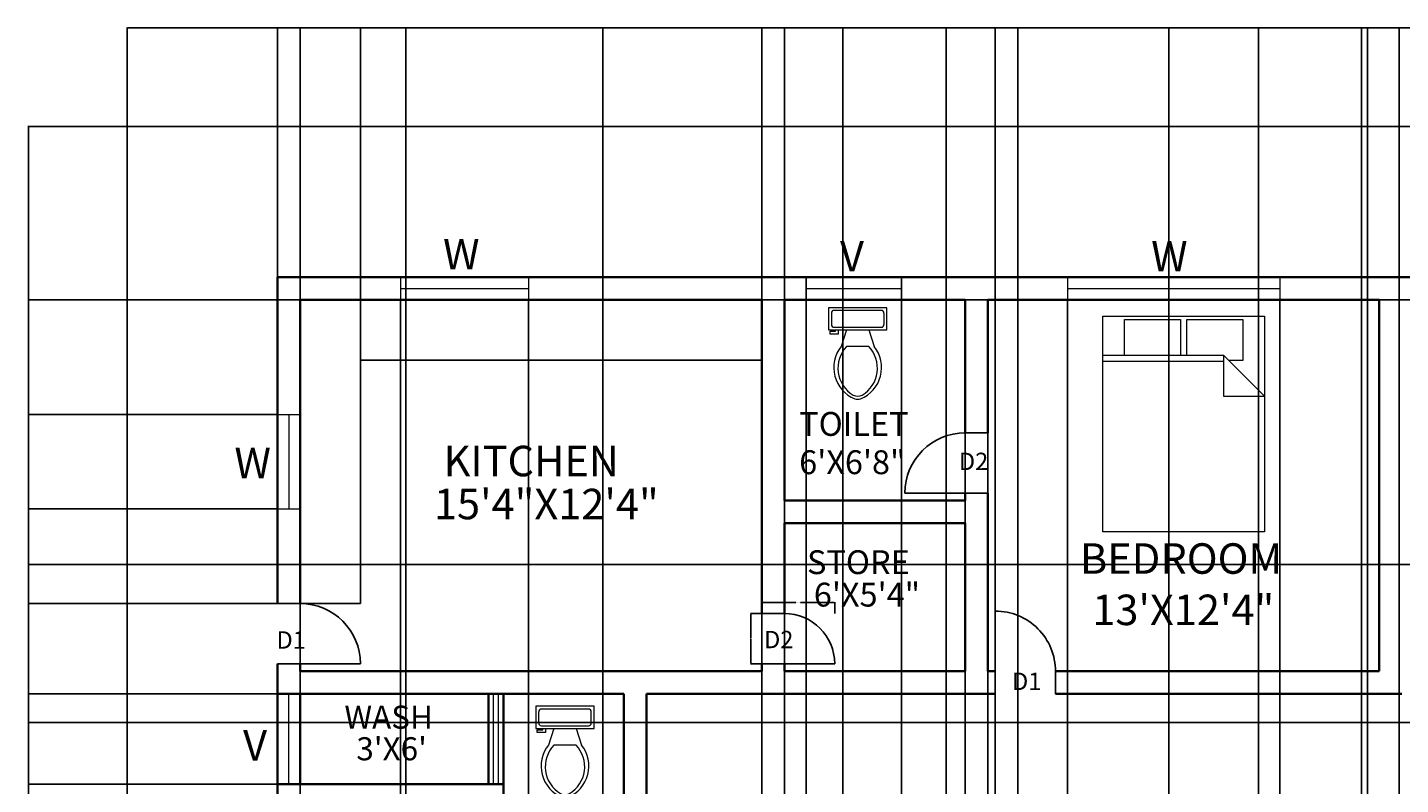
# Model space of a CAD drawing. Units: feet. Extents: x 2270 to 3094, y 1543 to 2352.
# Tile 5 of 6: x 2270 to 2817, y 2050 to 2352. Entities that reach past the tile are written whole.
import ezdxf

# ---------------------------------------------------------------- set-up
doc = ezdxf.new("R2010")
doc.units = ezdxf.units.FT
for name, color, linetype, lineweight in [('A-ANNO-DIMS', 2, 'Continuous', 18), ('A-ANNO-TEXT', 7, 'Continuous', 18), ('A-AREA-IDEN', 7, 'Continuous', 18), ('A-DOOR', 3, 'Continuous', 25), ('A-FLOR-CASE', 8, 'Continuous', 25), ('A-FLOR-FIXT', 8, 'Continuous', 18), ('A-FURN', 8, 'Continuous', 18), ('A-GLAZ', 4, 'Continuous', 18), ('A-WALL', 7, 'Continuous', 35), ('C-PROP', 8, 'Continuous', 25)]:
    doc.layers.add(name, color=color, linetype=linetype, lineweight=lineweight)
doc.styles.get("Standard").update_dxf_attribs({"font": 'arial.ttf'})
doc.dimstyles.get("Standard").update_dxf_attribs({"dimtxt": 0.18, "dimasz": 0.18, "dimexe": 0.18, "dimexo": 0.0625, "dimgap": 0.09, "dimtad": 0, "dimtih": 1, "dimtoh": 1, "dimdec": 4, "dimzin": 0, "dimdsep": 46, "dimtxsty": 'Standard', "dimcen": 0.09, "dimadec": 0, "dimazin": 0, "dimtfac": 1, "dimtdec": 4, "dimtofl": 0, "dimtmove": 0, "dimatfit": 3, "dimfxl": 1, "dimtolj": 1, "dimtzin": 0, "dimarcsym": 0})

# ---------------------------------------------------------------- blocks, each defined once
blk = doc.blocks.new('Bed - Queen')
for p, q in [((0, -80.00003), (0, 0)), ((0, 0), (59.99999, 0)), ((59.99999, 0), (59.99999, -80.00003)), ((7.99999, -1.2), (28.79998, -1.2)), ((7.99999, -14.4), (7.99999, -1.2)), ((28.79998, -1.2), (28.79998, -14.4)), ((31.19999, -1.2), (51.99999, -1.2)), ((31.19999, -14.4), (31.19999, -1.2)), ((51.99999, -1.2), (51.99999, -16.4)), ((0, -14.4), (44.8, -14.4)), ((59.99999, -29.6), (44.8, -14.4)), ((44.8, -14.4), (44.8, -29.6)), ((44.8, -16.8), (0, -16.8)), ((51.99999, -16.4), (46.79936, -16.4)), ((44.8, -29.6), (59.99999, -29.6)), ((59.99999, -80.00003), (0, -80.00003))]:
    blk.add_line(p, q)
blk = doc.blocks.new('Toilet - top')
for p, q in [((9.5, -6), (9.5, -2)), ((-10, -8.5), (-8, -8.5)), ((-10, -9.5), (-10, -8.5)), ((-7, -9.5), (-10, -9.5)), ((-8, -8.5), (-8, -8)), ((-7, -8), (-7, -9.5)), ((-4, -8), (-6, -14)), ((4, -8), (6, -14)), ((4, -14), (-4, -14))]:
    blk.add_line(p, q)
blk.add_lwpolyline([(10.5, -8), (10.5, 0), (-10.5, 0), (-10.5, -8)], close=True)
for points in [[(-9.5, -2), (-9.5, -6)], [(8.5, -1), (-8.5, -1)], [(-8.5, -7), (8.5, -7)]]:
    blk.add_lwpolyline(points)
for centre, radius, start, end in [((-8.62, -1.88), 0.884, 81.8699, 188.1301), ((8.62, -1.88), 0.884, 351.8699, 98.1301), ((-8.62, -6.12), 0.884, 171.8699, 278.1301), ((8.62, -6.12), 0.884, 261.8699, 8.1301), ((3.52, -21.58), 12.17, 141.4691, 247.9714), ((4.2, -21.82), 11.33, 136.3677, 238.9468), ((-3.52, -21.58), 12.17, 292.0284, 38.5307), ((-4.2, -21.82), 11.33, 301.053, 43.6321), ((0, -27.88), 4, 245.7318, 294.2682), ((0, -29), 4, 254.8605, 285.1395)]:
    blk.add_arc(centre, radius, start, end)
blk = doc.blocks.new('DOOR-SWING-24')
blk.add_line((33, 0), (0, 0))
blk.add_arc((9, 0), 24, 0, 90)
blk = doc.blocks.new('DOOR-SWING-20')
blk.add_line((0, 0), (29, 0))
blk.add_arc((9, 0), 20, 0, 90)
blk = doc.blocks.new('*D12')
at = {"layer": 'A-ANNO-DIMS', "color": 0, "lineweight": -2, "transparency": 16777216}
for p, q in [((2562.67, 2118.15), (2562.67, 2122.61)), ((2562.85, 2122.43), (2576.23, 2122.43)), ((2591.49, 2122.43), (2578.1, 2122.43)), ((2591.67, 2118.15), (2591.67, 2122.61))]:
    blk.add_line(p, q, dxfattribs=at)
at = {"layer": 'A-ANNO-DIMS', "color": 0, "transparency": 16777216}
for points in [[(2562.85, 2122.46), (2562.85, 2122.4), (2562.67, 2122.43)], [(2591.49, 2122.46), (2591.49, 2122.4), (2591.67, 2122.43)]]:
    blk.add_solid(points, dxfattribs=at)
at = {"layer": 'Defpoints', "color": 0, "transparency": 16777216}
for p in [(2562.67, 2118.08), (2591.67, 2122.43), (2591.67, 2118.08)]:
    blk.add_point(p, dxfattribs=at)
at = {"layer": 'A-ANNO-DIMS', "color": 0, "transparency": 16777216, "insert": (2577.17, 2122.43), "char_height": 0.18, "attachment_point": 5}
blk.add_mtext('\\A1;DOOR 29 TYP.', dxfattribs=at)
blk = doc.blocks.new('*D13')
at = {"layer": 'A-ANNO-DIMS', "color": 0, "lineweight": -2, "transparency": 16777216}
for p, q in [((2562.6, 2118.08), (2558.14, 2118.08)), ((2558.32, 2117.9), (2558.32, 2108.27)), ((2558.32, 2098.26), (2558.32, 2107.9)), ((2562.6, 2098.08), (2558.14, 2098.08))]:
    blk.add_line(p, q, dxfattribs=at)
at = {"layer": 'A-ANNO-DIMS', "color": 0, "transparency": 16777216}
for points in [[(2558.29, 2117.9), (2558.35, 2117.9), (2558.32, 2118.08)], [(2558.29, 2098.26), (2558.35, 2098.26), (2558.32, 2098.08)]]:
    blk.add_solid(points, dxfattribs=at)
at = {"layer": 'Defpoints', "color": 0, "transparency": 16777216}
for p in [(2558.32, 2118.08), (2562.67, 2118.08), (2562.67, 2098.08)]:
    blk.add_point(p, dxfattribs=at)
at = {"layer": 'A-ANNO-DIMS', "color": 0, "transparency": 16777216, "insert": (2558.32, 2108.08), "char_height": 0.18, "attachment_point": 5}
blk.add_mtext('\\A1;20 TYP.', dxfattribs=at)
blk = doc.blocks.new('*D26')
at = {"layer": 'A-ANNO-DIMS', "color": 0, "lineweight": -2, "transparency": 16777216}
for p, q in [((2309.67, 2312.15), (2309.67, 2351.56)), ((2309.85, 2351.38), (2681.88, 2351.38)), ((3054.49, 2351.38), (2682.45, 2351.38)), ((3054.67, 2312.15), (3054.67, 2351.56))]:
    blk.add_line(p, q, dxfattribs=at)
at = {"layer": 'A-ANNO-DIMS', "color": 0, "transparency": 16777216}
for points in [[(2309.85, 2351.41), (2309.85, 2351.35), (2309.67, 2351.38)], [(3054.49, 2351.41), (3054.49, 2351.35), (3054.67, 2351.38)]]:
    blk.add_solid(points, dxfattribs=at)
at = {"layer": 'Defpoints', "color": 0, "transparency": 16777216}
for p in [(3054.67, 2351.38), (2309.67, 2312.08), (3054.67, 2312.08)]:
    blk.add_point(p, dxfattribs=at)
at = {"layer": 'A-ANNO-DIMS', "color": 0, "transparency": 16777216, "insert": (2682.17, 2351.38), "char_height": 0.18, "attachment_point": 5}
blk.add_mtext('\\A1;745', dxfattribs=at)
blk = doc.blocks.new('*D27')
at = {"layer": 'A-ANNO-DIMS', "color": 0, "lineweight": -2, "transparency": 16777216}
for p, q in [((2309.6, 2312.08), (2270.19, 2312.08)), ((2270.37, 2311.9), (2270.37, 1963.27)), ((2270.37, 1614.26), (2270.37, 1962.9)), ((2309.6, 1614.08), (2270.19, 1614.08))]:
    blk.add_line(p, q, dxfattribs=at)
at = {"layer": 'A-ANNO-DIMS', "color": 0, "transparency": 16777216}
for points in [[(2270.34, 2311.9), (2270.4, 2311.9), (2270.37, 2312.08)], [(2270.34, 1614.26), (2270.4, 1614.26), (2270.37, 1614.08)]]:
    blk.add_solid(points, dxfattribs=at)
at = {"layer": 'Defpoints', "color": 0, "transparency": 16777216}
for p in [(2270.37, 2312.08), (2309.67, 2312.08), (2309.67, 1614.08)]:
    blk.add_point(p, dxfattribs=at)
at = {"layer": 'A-ANNO-DIMS', "color": 0, "transparency": 16777216, "insert": (2270.37, 1963.08), "char_height": 0.18, "attachment_point": 5}
blk.add_mtext('\\A1;698', dxfattribs=at)
blk = doc.blocks.new('*D30')
at = {"layer": 'A-ANNO-DIMS', "color": 0, "lineweight": -2, "transparency": 16777216}
for p, q in [((2369.67, 2252.15), (2369.67, 2351.56)), ((2369.85, 2351.38), (2681.88, 2351.38)), ((2994.49, 2351.38), (2682.46, 2351.38)), ((2994.67, 2252.15), (2994.67, 2351.56))]:
    blk.add_line(p, q, dxfattribs=at)
at = {"layer": 'A-ANNO-DIMS', "color": 0, "transparency": 16777216}
for points in [[(2369.85, 2351.41), (2369.85, 2351.35), (2369.67, 2351.38)], [(2994.49, 2351.41), (2994.49, 2351.35), (2994.67, 2351.38)]]:
    blk.add_solid(points, dxfattribs=at)
at = {"layer": 'Defpoints', "color": 0, "transparency": 16777216}
for p in [(2994.67, 2351.38), (2369.67, 2252.08), (2994.67, 2252.08)]:
    blk.add_point(p, dxfattribs=at)
at = {"layer": 'A-ANNO-DIMS', "color": 0, "transparency": 16777216, "insert": (2682.17, 2351.38), "char_height": 0.18, "attachment_point": 5}
blk.add_mtext('\\A1;625', dxfattribs=at)
blk = doc.blocks.new('*D32')
at = {"layer": 'A-ANNO-DIMS', "color": 0, "lineweight": -2, "transparency": 16777216}
for p, q in [((2378.67, 2243.02), (2378.67, 1574.6)), ((2418.6, 2243.02), (2418.6, 1574.6)), ((2378.85, 1574.78), (2398.24, 1574.78)), ((2418.42, 1574.78), (2399.02, 1574.78))]:
    blk.add_line(p, q, dxfattribs=at)
at = {"layer": 'A-ANNO-DIMS', "color": 0, "transparency": 16777216}
for points in [[(2378.85, 1574.81), (2378.85, 1574.75), (2378.67, 1574.78)], [(2418.42, 1574.81), (2418.42, 1574.75), (2418.6, 1574.78)]]:
    blk.add_solid(points, dxfattribs=at)
at = {"layer": 'Defpoints', "color": 0, "transparency": 16777216}
for p in [(2378.67, 2243.08), (2418.6, 2243.08), (2418.6, 1574.78)]:
    blk.add_point(p, dxfattribs=at)
at = {"layer": 'A-ANNO-DIMS', "color": 0, "transparency": 16777216, "insert": (2398.63, 1574.78), "char_height": 0.18, "attachment_point": 5}
blk.add_mtext('\\A1;39.93', dxfattribs=at)
blk = doc.blocks.new('*D33')
at = {"layer": 'A-ANNO-DIMS', "color": 0, "lineweight": -2, "transparency": 16777216}
for p, q in [((2418.6, 2243.02), (2418.6, 1574.6)), ((2469.65, 2243.02), (2469.65, 1574.6)), ((2418.78, 1574.78), (2443.73, 1574.78)), ((2469.47, 1574.78), (2444.52, 1574.78))]:
    blk.add_line(p, q, dxfattribs=at)
at = {"layer": 'A-ANNO-DIMS', "color": 0, "transparency": 16777216}
for points in [[(2418.78, 1574.81), (2418.78, 1574.75), (2418.6, 1574.78)], [(2469.47, 1574.81), (2469.47, 1574.75), (2469.65, 1574.78)]]:
    blk.add_solid(points, dxfattribs=at)
at = {"layer": 'Defpoints', "color": 0, "transparency": 16777216}
for p in [(2418.6, 2243.08), (2469.65, 2243.08), (2469.65, 1574.78)]:
    blk.add_point(p, dxfattribs=at)
at = {"layer": 'A-ANNO-DIMS', "color": 0, "transparency": 16777216, "insert": (2444.12, 1574.78), "char_height": 0.18, "attachment_point": 5}
blk.add_mtext('\\A1;51.05', dxfattribs=at)
blk = doc.blocks.new('*D34')
at = {"layer": 'A-ANNO-DIMS', "color": 0, "lineweight": -2, "transparency": 16777216}
for p, q in [((2580.32, 2252.02), (2580.32, 1574.6)), ((2618.3, 2252.02), (2618.3, 1574.6)), ((2580.5, 1574.78), (2598.92, 1574.78)), ((2618.12, 1574.78), (2599.7, 1574.78))]:
    blk.add_line(p, q, dxfattribs=at)
at = {"layer": 'A-ANNO-DIMS', "color": 0, "transparency": 16777216}
for points in [[(2580.5, 1574.81), (2580.5, 1574.75), (2580.32, 1574.78)], [(2618.12, 1574.81), (2618.12, 1574.75), (2618.3, 1574.78)]]:
    blk.add_solid(points, dxfattribs=at)
at = {"layer": 'Defpoints', "color": 0, "transparency": 16777216}
for p in [(2580.32, 2252.08), (2618.3, 2252.08), (2618.3, 1574.78)]:
    blk.add_point(p, dxfattribs=at)
at = {"layer": 'A-ANNO-DIMS', "color": 0, "transparency": 16777216, "insert": (2599.31, 1574.78), "char_height": 0.18, "attachment_point": 5}
blk.add_mtext('\\A1;37.98', dxfattribs=at)
blk = doc.blocks.new('*D35')
at = {"layer": 'A-ANNO-DIMS', "color": 0, "lineweight": -2, "transparency": 16777216}
for p, q in [((2618.3, 2243.02), (2618.3, 1574.6)), ((2643.67, 2243.02), (2643.67, 1574.6)), ((2618.48, 1574.78), (2630.52, 1574.78)), ((2643.49, 1574.78), (2631.45, 1574.78))]:
    blk.add_line(p, q, dxfattribs=at)
at = {"layer": 'A-ANNO-DIMS', "color": 0, "transparency": 16777216}
for points in [[(2618.48, 1574.81), (2618.48, 1574.75), (2618.3, 1574.78)], [(2643.49, 1574.81), (2643.49, 1574.75), (2643.67, 1574.78)]]:
    blk.add_solid(points, dxfattribs=at)
at = {"layer": 'Defpoints', "color": 0, "transparency": 16777216}
for p in [(2618.3, 2243.08), (2643.67, 2243.08), (2643.67, 1574.78)]:
    blk.add_point(p, dxfattribs=at)
at = {"layer": 'A-ANNO-DIMS', "color": 0, "transparency": 16777216, "insert": (2630.98, 1574.78), "char_height": 0.18, "attachment_point": 5}
blk.add_mtext('\\A1;25.366', dxfattribs=at)
blk = doc.blocks.new('*D36')
at = {"layer": 'A-ANNO-DIMS', "color": 0, "lineweight": -2, "transparency": 16777216}
for p, q in [((2652.67, 2243.02), (2652.67, 1574.6)), ((2684.42, 2243.02), (2684.42, 1574.6)), ((2652.85, 1574.78), (2668.15, 1574.78)), ((2684.24, 1574.78), (2668.94, 1574.78))]:
    blk.add_line(p, q, dxfattribs=at)
at = {"layer": 'A-ANNO-DIMS', "color": 0, "transparency": 16777216}
for points in [[(2652.85, 1574.81), (2652.85, 1574.75), (2652.67, 1574.78)], [(2684.24, 1574.81), (2684.24, 1574.75), (2684.42, 1574.78)]]:
    blk.add_solid(points, dxfattribs=at)
at = {"layer": 'Defpoints', "color": 0, "transparency": 16777216}
for p in [(2652.67, 2243.08), (2684.42, 2243.08), (2684.42, 1574.78)]:
    blk.add_point(p, dxfattribs=at)
at = {"layer": 'A-ANNO-DIMS', "color": 0, "transparency": 16777216, "insert": (2668.55, 1574.78), "char_height": 0.18, "attachment_point": 5}
blk.add_mtext('\\A1;31.76', dxfattribs=at)
blk = doc.blocks.new('*D37')
at = {"layer": 'A-ANNO-DIMS', "color": 0, "lineweight": -2, "transparency": 16777216}
for p, q in [((2684.42, 2243.02), (2684.42, 1574.6)), ((2769.01, 2243.02), (2769.01, 1574.6)), ((2684.6, 1574.78), (2726.32, 1574.78)), ((2768.83, 1574.78), (2727.11, 1574.78))]:
    blk.add_line(p, q, dxfattribs=at)
at = {"layer": 'A-ANNO-DIMS', "color": 0, "transparency": 16777216}
for points in [[(2684.6, 1574.81), (2684.6, 1574.75), (2684.42, 1574.78)], [(2768.83, 1574.81), (2768.83, 1574.75), (2769.01, 1574.78)]]:
    blk.add_solid(points, dxfattribs=at)
at = {"layer": 'Defpoints', "color": 0, "transparency": 16777216}
for p in [(2684.42, 2243.08), (2769.01, 2243.08), (2769.01, 1574.78)]:
    blk.add_point(p, dxfattribs=at)
at = {"layer": 'A-ANNO-DIMS', "color": 0, "transparency": 16777216, "insert": (2726.71, 1574.78), "char_height": 0.18, "attachment_point": 5}
blk.add_mtext('\\A1;84.58', dxfattribs=at)
blk = doc.blocks.new('*D40')
at = {"layer": 'A-ANNO-DIMS', "color": 0, "lineweight": -2, "transparency": 16777216}
for p, q in [((2985.6, 2243.08), (2270.19, 2243.08)), ((2270.37, 2242.9), (2270.37, 2190.53)), ((2270.37, 2137.79), (2270.37, 2190.16)), ((2985.6, 2137.61), (2270.19, 2137.61))]:
    blk.add_line(p, q, dxfattribs=at)
at = {"layer": 'A-ANNO-DIMS', "color": 0, "transparency": 16777216}
for points in [[(2270.34, 2242.9), (2270.4, 2242.9), (2270.37, 2243.08)], [(2270.34, 2137.79), (2270.4, 2137.79), (2270.37, 2137.61)]]:
    blk.add_solid(points, dxfattribs=at)
at = {"layer": 'Defpoints', "color": 0, "transparency": 16777216}
for p in [(2985.67, 2243.08), (2270.37, 2137.61), (2985.67, 2137.61)]:
    blk.add_point(p, dxfattribs=at)
at = {"layer": 'A-ANNO-DIMS', "color": 0, "transparency": 16777216, "insert": (2270.37, 2190.35), "char_height": 0.18, "attachment_point": 5}
blk.add_mtext('\\A1;105.48', dxfattribs=at)
blk = doc.blocks.new('*D41')
at = {"layer": 'A-ANNO-DIMS', "color": 0, "lineweight": -2, "transparency": 16777216}
for p, q in [((2985.6, 2137.61), (2270.19, 2137.61)), ((2270.37, 2137.43), (2270.37, 2106.32)), ((2270.37, 2074.84), (2270.37, 2105.95)), ((2985.6, 2074.66), (2270.19, 2074.66))]:
    blk.add_line(p, q, dxfattribs=at)
at = {"layer": 'A-ANNO-DIMS', "color": 0, "transparency": 16777216}
for points in [[(2270.34, 2137.43), (2270.4, 2137.43), (2270.37, 2137.61)], [(2270.34, 2074.84), (2270.4, 2074.84), (2270.37, 2074.66)]]:
    blk.add_solid(points, dxfattribs=at)
at = {"layer": 'Defpoints', "color": 0, "transparency": 16777216}
for p in [(2985.67, 2137.61), (2270.37, 2074.66), (2985.67, 2074.66)]:
    blk.add_point(p, dxfattribs=at)
at = {"layer": 'A-ANNO-DIMS', "color": 0, "transparency": 16777216, "insert": (2270.37, 2106.14), "char_height": 0.18, "attachment_point": 5}
blk.add_mtext('\\A1;62.94', dxfattribs=at)
blk = doc.blocks.new('*D47')
at = {"layer": 'A-ANNO-DIMS', "color": 0, "lineweight": -2, "transparency": 16777216}
for p, q in [((2760.54, 1820.15), (2760.54, 2351.56)), ((2760.72, 2351.38), (2788.21, 2351.38)), ((2816.49, 2351.38), (2788.99, 2351.38)), ((2816.67, 1820.15), (2816.67, 2351.56))]:
    blk.add_line(p, q, dxfattribs=at)
at = {"layer": 'A-ANNO-DIMS', "color": 0, "transparency": 16777216}
for points in [[(2760.72, 2351.41), (2760.72, 2351.35), (2760.54, 2351.38)], [(2816.49, 2351.41), (2816.49, 2351.35), (2816.67, 2351.38)]]:
    blk.add_solid(points, dxfattribs=at)
at = {"layer": 'Defpoints', "color": 0, "transparency": 16777216}
for p in [(2816.67, 2351.38), (2760.54, 1820.08), (2816.67, 1820.08)]:
    blk.add_point(p, dxfattribs=at)
at = {"layer": 'A-ANNO-DIMS', "color": 0, "transparency": 16777216, "insert": (2788.6, 2351.38), "char_height": 0.18, "attachment_point": 5}
blk.add_mtext('\\A1;56.13', dxfattribs=at)
blk = doc.blocks.new('*D48')
at = {"layer": 'A-ANNO-DIMS', "color": 0, "lineweight": -2, "transparency": 16777216}
for p, q in [((2664.67, 1698.15), (2664.67, 2351.56)), ((2664.85, 2351.38), (2732.89, 2351.38)), ((2801.49, 2351.38), (2733.45, 2351.38)), ((2801.67, 1698.15), (2801.67, 2351.56))]:
    blk.add_line(p, q, dxfattribs=at)
at = {"layer": 'A-ANNO-DIMS', "color": 0, "transparency": 16777216}
for points in [[(2664.85, 2351.41), (2664.85, 2351.35), (2664.67, 2351.38)], [(2801.49, 2351.41), (2801.49, 2351.35), (2801.67, 2351.38)]]:
    blk.add_solid(points, dxfattribs=at)
at = {"layer": 'Defpoints', "color": 0, "transparency": 16777216}
for p in [(2801.67, 2351.38), (2664.67, 1698.08), (2801.67, 1698.08)]:
    blk.add_point(p, dxfattribs=at)
at = {"layer": 'A-ANNO-DIMS', "color": 0, "transparency": 16777216, "insert": (2733.17, 2351.38), "char_height": 0.18, "attachment_point": 5}
blk.add_mtext('\\A1;137', dxfattribs=at)
blk = doc.blocks.new('*D50')
at = {"layer": 'A-ANNO-DIMS', "color": 0, "lineweight": -2, "transparency": 16777216}
for p, q in [((2378.67, 1683.15), (2378.67, 2351.56)), ((2378.85, 2351.38), (2399.3, 2351.38)), ((2420.55, 2351.38), (2400.1, 2351.38)), ((2420.73, 1683.15), (2420.73, 2351.56))]:
    blk.add_line(p, q, dxfattribs=at)
at = {"layer": 'A-ANNO-DIMS', "color": 0, "transparency": 16777216}
for points in [[(2378.85, 2351.41), (2378.85, 2351.35), (2378.67, 2351.38)], [(2420.55, 2351.41), (2420.55, 2351.35), (2420.73, 2351.38)]]:
    blk.add_solid(points, dxfattribs=at)
at = {"layer": 'Defpoints', "color": 0, "transparency": 16777216}
for p in [(2420.73, 2351.38), (2378.67, 1683.08), (2420.73, 1683.08)]:
    blk.add_point(p, dxfattribs=at)
at = {"layer": 'A-ANNO-DIMS', "color": 0, "transparency": 16777216, "insert": (2399.7, 2351.38), "char_height": 0.18, "attachment_point": 5}
blk.add_mtext('\\A1;42.07', dxfattribs=at)
blk = doc.blocks.new('*D51')
at = {"layer": 'A-ANNO-DIMS', "color": 0, "lineweight": -2, "transparency": 16777216}
for p, q in [((2420.73, 1683.15), (2420.73, 2351.56)), ((2420.91, 2351.38), (2459.61, 2351.38)), ((2499.1, 2351.38), (2460.4, 2351.38)), ((2499.28, 1683.15), (2499.28, 2351.56))]:
    blk.add_line(p, q, dxfattribs=at)
at = {"layer": 'A-ANNO-DIMS', "color": 0, "transparency": 16777216}
for points in [[(2420.91, 2351.41), (2420.91, 2351.35), (2420.73, 2351.38)], [(2499.1, 2351.41), (2499.1, 2351.35), (2499.28, 2351.38)]]:
    blk.add_solid(points, dxfattribs=at)
at = {"layer": 'Defpoints', "color": 0, "transparency": 16777216}
for p in [(2499.28, 2351.38), (2420.73, 1683.08), (2499.28, 1683.08)]:
    blk.add_point(p, dxfattribs=at)
at = {"layer": 'A-ANNO-DIMS', "color": 0, "transparency": 16777216, "insert": (2460.01, 2351.38), "char_height": 0.18, "attachment_point": 5}
blk.add_mtext('\\A1;78.55', dxfattribs=at)
blk = doc.blocks.new('*D52')
at = {"layer": 'A-ANNO-DIMS', "color": 0, "lineweight": -2, "transparency": 16777216}
for p, q in [((2594.98, 1683.15), (2594.98, 2351.56)), ((2595.16, 2351.38), (2615.09, 2351.38)), ((2635.97, 2351.38), (2616.03, 2351.38)), ((2636.15, 1683.15), (2636.15, 2351.56))]:
    blk.add_line(p, q, dxfattribs=at)
at = {"layer": 'A-ANNO-DIMS', "color": 0, "transparency": 16777216}
for points in [[(2595.16, 2351.41), (2595.16, 2351.35), (2594.98, 2351.38)], [(2635.97, 2351.41), (2635.97, 2351.35), (2636.15, 2351.38)]]:
    blk.add_solid(points, dxfattribs=at)
at = {"layer": 'Defpoints', "color": 0, "transparency": 16777216}
for p in [(2636.15, 2351.38), (2594.98, 1683.08), (2636.15, 1683.08)]:
    blk.add_point(p, dxfattribs=at)
at = {"layer": 'A-ANNO-DIMS', "color": 0, "transparency": 16777216, "insert": (2615.56, 2351.38), "char_height": 0.18, "attachment_point": 5}
blk.add_mtext('\\A1;41.175', dxfattribs=at)
blk = doc.blocks.new('*D53')
at = {"layer": 'A-ANNO-DIMS', "color": 0, "lineweight": -2, "transparency": 16777216}
for p, q in [((2636.15, 1683.15), (2636.15, 2351.56)), ((2636.33, 2351.38), (2645.45, 2351.38)), ((2655.49, 2351.38), (2646.36, 2351.38)), ((2655.67, 1683.15), (2655.67, 2351.56))]:
    blk.add_line(p, q, dxfattribs=at)
at = {"layer": 'A-ANNO-DIMS', "color": 0, "transparency": 16777216}
for points in [[(2636.33, 2351.41), (2636.33, 2351.35), (2636.15, 2351.38)], [(2655.49, 2351.41), (2655.49, 2351.35), (2655.67, 2351.38)]]:
    blk.add_solid(points, dxfattribs=at)
at = {"layer": 'Defpoints', "color": 0, "transparency": 16777216}
for p in [(2655.67, 2351.38), (2636.15, 1683.08), (2655.67, 1683.08)]:
    blk.add_point(p, dxfattribs=at)
at = {"layer": 'A-ANNO-DIMS', "color": 0, "transparency": 16777216, "insert": (2645.91, 2351.38), "char_height": 0.18, "attachment_point": 5}
blk.add_mtext('\\A1;19.516', dxfattribs=at)
blk = doc.blocks.new('*D58')
at = {"layer": 'A-ANNO-DIMS', "color": 0, "lineweight": -2, "transparency": 16777216}
for p, q in [((2369.6, 2086.08), (2270.19, 2086.08)), ((2270.37, 2085.9), (2270.37, 2068.27)), ((2270.37, 2050.26), (2270.37, 2067.9)), ((2369.6, 2050.08), (2270.19, 2050.08))]:
    blk.add_line(p, q, dxfattribs=at)
at = {"layer": 'A-ANNO-DIMS', "color": 0, "transparency": 16777216}
for points in [[(2270.34, 2085.9), (2270.4, 2085.9), (2270.37, 2086.08)], [(2270.34, 2050.26), (2270.4, 2050.26), (2270.37, 2050.08)]]:
    blk.add_solid(points, dxfattribs=at)
at = {"layer": 'Defpoints', "color": 0, "transparency": 16777216}
for p in [(2270.37, 2086.08), (2369.67, 2086.08), (2369.67, 2050.08)]:
    blk.add_point(p, dxfattribs=at)
at = {"layer": 'A-ANNO-DIMS', "color": 0, "transparency": 16777216, "insert": (2270.37, 2068.08), "char_height": 0.18, "attachment_point": 5}
blk.add_mtext('\\A1;36', dxfattribs=at)
blk = doc.blocks.new('*D59')
at = {"layer": 'A-ANNO-DIMS', "color": 0, "lineweight": -2, "transparency": 16777216}
for p, q in [((2369.6, 2159.8), (2270.19, 2159.8)), ((2270.37, 2159.62), (2270.37, 2141.13)), ((2270.37, 2122.26), (2270.37, 2140.76)), ((2369.6, 2122.08), (2270.19, 2122.08))]:
    blk.add_line(p, q, dxfattribs=at)
at = {"layer": 'A-ANNO-DIMS', "color": 0, "transparency": 16777216}
for points in [[(2270.34, 2159.62), (2270.4, 2159.62), (2270.37, 2159.8)], [(2270.34, 2122.26), (2270.4, 2122.26), (2270.37, 2122.08)]]:
    blk.add_solid(points, dxfattribs=at)
at = {"layer": 'Defpoints', "color": 0, "transparency": 16777216}
for p in [(2270.37, 2159.8), (2369.67, 2159.8), (2369.67, 2122.08)]:
    blk.add_point(p, dxfattribs=at)
at = {"layer": 'A-ANNO-DIMS', "color": 0, "transparency": 16777216, "insert": (2270.37, 2140.94), "char_height": 0.18, "attachment_point": 5}
blk.add_mtext('\\A1;37.72', dxfattribs=at)
blk = doc.blocks.new('*D60')
at = {"layer": 'A-ANNO-DIMS', "color": 0, "lineweight": -2, "transparency": 16777216}
for p, q in [((2369.6, 2197.41), (2270.19, 2197.41)), ((2270.37, 2197.23), (2270.37, 2178.79)), ((2270.37, 2159.98), (2270.37, 2178.42)), ((2369.6, 2159.8), (2270.19, 2159.8))]:
    blk.add_line(p, q, dxfattribs=at)
at = {"layer": 'A-ANNO-DIMS', "color": 0, "transparency": 16777216}
for points in [[(2270.34, 2197.23), (2270.4, 2197.23), (2270.37, 2197.41)], [(2270.34, 2159.98), (2270.4, 2159.98), (2270.37, 2159.8)]]:
    blk.add_solid(points, dxfattribs=at)
at = {"layer": 'Defpoints', "color": 0, "transparency": 16777216}
for p in [(2270.37, 2197.41), (2369.67, 2197.41), (2369.67, 2159.8)]:
    blk.add_point(p, dxfattribs=at)
at = {"layer": 'A-ANNO-DIMS', "color": 0, "transparency": 16777216, "insert": (2270.37, 2178.61), "char_height": 0.18, "attachment_point": 5}
blk.add_mtext('\\A1;37.604', dxfattribs=at)
blk = doc.blocks.new('*D64')
at = {"layer": 'A-ANNO-DIMS', "color": 0, "lineweight": -2, "transparency": 16777216}
for p, q in [((2378.67, 2122.15), (2378.67, 2351.56)), ((2378.85, 2351.38), (2390.45, 2351.38)), ((2402.49, 2351.38), (2390.89, 2351.38)), ((2402.67, 2122.15), (2402.67, 2351.56))]:
    blk.add_line(p, q, dxfattribs=at)
at = {"layer": 'A-ANNO-DIMS', "color": 0, "transparency": 16777216}
for points in [[(2378.85, 2351.41), (2378.85, 2351.35), (2378.67, 2351.38)], [(2402.49, 2351.41), (2402.49, 2351.35), (2402.67, 2351.38)]]:
    blk.add_solid(points, dxfattribs=at)
at = {"layer": 'Defpoints', "color": 0, "transparency": 16777216}
for p in [(2402.67, 2351.38), (2378.67, 2122.08), (2402.67, 2122.08)]:
    blk.add_point(p, dxfattribs=at)
at = {"layer": 'A-ANNO-DIMS', "color": 0, "transparency": 16777216, "insert": (2390.67, 2351.38), "char_height": 0.18, "attachment_point": 5}
blk.add_mtext('\\A1;24', dxfattribs=at)
blk = doc.blocks.new('*D65')
at = {"layer": 'A-ANNO-DIMS', "color": 0, "lineweight": -2, "transparency": 16777216}
for p, q in [((2562.67, 1683.15), (2562.67, 2351.56)), ((2562.85, 2351.38), (2567.02, 2351.38)), ((2571.49, 2351.38), (2567.32, 2351.38)), ((2571.67, 1683.15), (2571.67, 2351.56))]:
    blk.add_line(p, q, dxfattribs=at)
at = {"layer": 'A-ANNO-DIMS', "color": 0, "transparency": 16777216}
for points in [[(2562.85, 2351.41), (2562.85, 2351.35), (2562.67, 2351.38)], [(2571.49, 2351.41), (2571.49, 2351.35), (2571.67, 2351.38)]]:
    blk.add_solid(points, dxfattribs=at)
at = {"layer": 'Defpoints', "color": 0, "transparency": 16777216}
for p in [(2571.67, 2351.38), (2562.67, 1683.08), (2571.67, 1683.08)]:
    blk.add_point(p, dxfattribs=at)
at = {"layer": 'A-ANNO-DIMS', "color": 0, "transparency": 16777216, "insert": (2567.17, 2351.38), "char_height": 0.18, "attachment_point": 5}
blk.add_mtext('\\A1;9', dxfattribs=at)
blk = doc.blocks.new('*D66')
at = {"layer": 'A-ANNO-DIMS', "color": 0, "lineweight": -2, "transparency": 16777216}
for p, q in [((2724.84, 1977.15), (2724.84, 2351.56)), ((2725.02, 2351.38), (2764.01, 2351.38)), ((2803.78, 2351.38), (2764.79, 2351.38)), ((2803.96, 1977.15), (2803.96, 2351.56))]:
    blk.add_line(p, q, dxfattribs=at)
at = {"layer": 'A-ANNO-DIMS', "color": 0, "transparency": 16777216}
for points in [[(2725.02, 2351.41), (2725.02, 2351.35), (2724.84, 2351.38)], [(2803.78, 2351.41), (2803.78, 2351.35), (2803.96, 2351.38)]]:
    blk.add_solid(points, dxfattribs=at)
at = {"layer": 'Defpoints', "color": 0, "transparency": 16777216}
for p in [(2803.96, 2351.38), (2724.84, 1977.08), (2803.96, 1977.08)]:
    blk.add_point(p, dxfattribs=at)
at = {"layer": 'A-ANNO-DIMS', "color": 0, "transparency": 16777216, "insert": (2764.4, 2351.38), "char_height": 0.18, "attachment_point": 5}
blk.add_mtext('\\A1;79.12', dxfattribs=at)

msp = doc.modelspace()

# ---------------------------------------------------------------- linework, layer by layer
at = {"layer": 'A-DOOR'}
for p, q in [((2652.6659, 2190.0845), (2643.6659, 2190.0845)), ((2562.6659, 2118.0845), (2571.6659, 2118.0845)), ((2679.6659, 2095.0845), (2679.6659, 2086.0845))]:
    msp.add_line(p, q, dxfattribs=at)
at = {"layer": 'A-FLOR-CASE'}
for p, q in [((2402.6659, 2219.0845), (2562.6659, 2219.0845)), ((2402.6659, 2122.0845), (2402.6659, 2219.0845)), ((2402.6659, 2122.0845), (2369.6659, 2122.0845))]:
    msp.add_line(p, q, dxfattribs=at)
at = {"layer": 'A-GLAZ'}
for p, q in [((2418.5967, 2252.0845), (2418.5967, 2243.0845)), ((2469.6502, 2252.0845), (2469.6502, 2243.0845)), ((2580.3205, 2252.0845), (2580.3205, 2243.0845)), ((2618.2997, 2252.0845), (2618.2997, 2243.0845)), ((2684.4243, 2252.0845), (2684.4243, 2243.0845)), ((2769.0053, 2252.0845), (2769.0053, 2243.0845)), ((2418.5967, 2247.5845), (2469.6502, 2247.5845)), ((2580.3205, 2247.5845), (2618.2997, 2247.5845)), ((2684.4243, 2247.5845), (2769.0053, 2247.5845)), ((2369.6659, 2197.4087), (2378.6659, 2197.4087)), ((2374.1659, 2197.4087), (2374.1659, 2159.8044)), ((2369.6659, 2159.8044), (2378.6659, 2159.8044)), ((2374.1659, 2050.0845), (2374.1659, 2086.0845)), ((2455.6659, 2050.0845), (2455.6659, 2086.0845)), ((2457.6659, 2050.0845), (2457.6659, 2086.0845))]:
    msp.add_line(p, q, dxfattribs=at)
at = {"layer": 'A-WALL'}
for p, q in [((2369.6659, 2252.0845), (2562.6659, 2252.0845)), ((2369.6659, 2252.0845), (2994.6659, 2252.0845)), ((2369.6659, 2252.0845), (2369.6659, 2122.0845)), ((2369.6659, 2122.0845), (2369.6659, 2252.0845)), ((2571.6659, 2252.0845), (2643.6659, 2252.0845)), ((2652.6659, 2252.0845), (2808.6659, 2252.0845)), ((2378.6659, 2243.0845), (2562.6659, 2243.0845)), ((2378.6659, 2122.0845), (2378.6659, 2243.0845)), ((2562.6659, 2243.0845), (2562.6659, 2118.0845)), ((2571.6659, 2243.0845), (2571.6659, 2163.0845)), ((2571.6659, 2243.0845), (2643.6659, 2243.0845)), ((2643.6659, 2243.0845), (2643.6659, 2190.0845)), ((2652.6659, 2243.0845), (2652.6659, 2190.0845)), ((2652.6659, 2243.0845), (2808.6659, 2243.0845)), ((2808.6659, 2243.0845), (2808.6659, 2095.0845)), ((2637.6659, 2163.0845), (2571.6659, 2163.0845)), ((2643.6659, 2163.0845), (2637.6659, 2163.0845)), ((2643.6659, 2166.0845), (2643.6659, 2163.0845)), ((2652.6659, 2166.0845), (2652.6659, 2095.0845)), ((2643.6659, 2154.0845), (2571.6659, 2154.0845)), ((2571.6659, 2154.0845), (2571.6659, 2118.0845)), ((2643.6659, 2154.0845), (2643.6659, 2095.0845)), ((2652.6659, 2154.0845), (2652.6659, 2095.0845)), ((2369.6659, 2095.0845), (2369.6659, 2098.0845)), ((2369.6659, 2098.0845), (2369.6659, 1674.0845)), ((2378.6659, 2095.0845), (2378.6659, 2098.0845)), ((2562.6659, 2098.0845), (2562.6659, 2095.0845)), ((2571.6659, 2098.0845), (2571.6659, 2095.0845)), ((2808.6659, 2095.0845), (2808.6659, 2098.6012)), ((2562.6659, 2095.0845), (2378.6659, 2095.0845)), ((2571.6659, 2095.0845), (2643.6659, 2095.0845)), ((2655.6659, 2095.0845), (2652.6659, 2095.0845)), ((2808.6659, 2095.0845), (2679.6659, 2095.0845)), ((2369.6659, 2086.0845), (2369.6659, 2050.0845)), ((2459.6659, 2086.0845), (2369.6659, 2086.0845)), ((2378.6659, 2086.0845), (2378.6659, 2050.0845)), ((2453.6659, 2050.0845), (2453.6659, 2086.0845)), ((2459.6659, 2086.0845), (2507.6659, 2086.0845)), ((2459.6659, 2050.0845), (2459.6659, 2086.0845)), ((2507.6659, 2086.0845), (2507.6659, 2000.0845)), ((2516.6659, 2086.0845), (2516.6659, 2000.0845)), ((2655.6659, 2086.0845), (2516.6659, 2086.0845)), ((2571.6659, 2086.0845), (2643.6659, 2086.0845)), ((2817.6659, 2086.0845), (2679.6659, 2086.0845)), ((2369.6659, 2050.0845), (2459.6659, 2050.0845)), ((2459.6659, 1977.0845), (2459.6659, 2050.0845))]:
    msp.add_line(p, q, dxfattribs=at)
at = {"layer": 'C-PROP'}
for p, q in [((2369.6659, 2312.0845), (2309.6659, 2312.0845)), ((2309.6659, 2312.0845), (2309.6659, 1614.0845)), ((3054.6659, 2312.0845), (2369.6659, 2312.0845))]:
    msp.add_line(p, q, dxfattribs=at)

# ---------------------------------------------------------------- block references
at = {"layer": 'A-DOOR', "extrusion": (0, 0, -1), "zscale": -1}
msp.add_blockref('DOOR-SWING-24', (-2652.6658, 2166.085), dxfattribs=at)
at = {"layer": 'A-DOOR'}
for name, p in [('DOOR-SWING-24', (2369.666, 2098.085)), ('DOOR-SWING-20', (2562.666, 2098.085))]:
    msp.add_blockref(name, p, dxfattribs=at)
at = {"layer": 'A-DOOR', "extrusion": (0, 0, -1), "zscale": -1, "rotation": 89.99999999999699}
msp.add_blockref('DOOR-SWING-24', (-2655.6664, 2086.0846), dxfattribs=at)
at = {"layer": 'A-FLOR-FIXT', "xscale": 1.103431246609896, "yscale": 1.103431246609896, "zscale": 1.103431246609896}
for p in [(2600.8464, 2239.8994), (2484.1878, 2081.1448)]:
    msp.add_blockref('Toilet - top', p, dxfattribs=at)
at = {"layer": 'A-FURN', "xscale": 1.073910050689623, "yscale": 1.073910050689623, "zscale": 1.073910050689623}
msp.add_blockref('Bed - Queen', (2698.5264, 2236.5066), dxfattribs=at)

# ---------------------------------------------------------------- texts
at = {"layer": 'A-ANNO-TEXT'}
for s, height, p in [('W', 12.1456, (2435.5991, 2255.1591)), ('V', 12.1456, (2593.7992, 2254.3742)), ('W', 12.1456, (2717.7752, 2254.3959)), ('W', 12.1456, (2352.4674, 2171.9782)), ('D2', 6.89564, (2641.1658, 2175.2663)), ('D1', 6.89564, (2369.2385, 2104.1121)), ('D2', 6.89564, (2563.5338, 2104.2863)), ('D1', 6.89564, (2662.347, 2087.6461)), ('V', 12.1456, (2355.9153, 2059.5506))]:
    msp.add_text(s, height=height, dxfattribs=at).set_placement(p)
at = {"layer": 'A-AREA-IDEN'}
for s, height, p in [('TOILET', 9.49664, (2577.5258, 2188.8802)), ('KITCHEN', 12.14556, (2435.8159, 2172.7799)), ('6\'X6\'8"', 9.49664, (2577.5258, 2173.6247)), ('15\'4"X12\'4"', 12.145557, (2431.9608, 2155.6506)), ('BEDROOM', 12.14556, (2689.4142, 2133.9297)), ('STORE', 9.49664, (2580.6438, 2133.8074)), ('6\'X5\'4"', 9.49664, (2583.368, 2120.8749)), ('13\'X12\'4"', 12.14556, (2694.3191, 2113.4854)), ('WASH', 9.20351, (2396.296, 2072.2076)), ("3'X6'", 9.20351, (2401.0508, 2059.6225))]:
    msp.add_text(s, height=height, dxfattribs=at).set_placement(p)

# ---------------------------------------------------------------- dimensions: what is measured, and where the dimension line sits
at = {"layer": 'A-ANNO-DIMS'}
for base, p1, p2, override, picture, middle in [((3054.6659, 2351.3845), (2309.6659, 2312.0845), (3054.6659, 2312.0845), {"dimdec": 0, "dimlfac": 1, "dimrnd": 0, "dimzin": 0, "dimdsep": 46, "dimlunit": 2}, '*D26', (2682.1659, 2351.3845)), ((2994.6659, 2351.3845), (2369.6659, 2252.0845), (2994.6659, 2252.0845), {"dimdec": 0, "dimlfac": 1, "dimrnd": 0, "dimzin": 0, "dimdsep": 46, "dimlunit": 2}, '*D30', (2682.1659, 2351.3845)), ((2420.7322, 2351.3845), (2378.6659, 1683.0845), (2420.7322, 1683.0845), {"dimdec": 2, "dimlfac": 1, "dimrnd": 0, "dimzin": 0, "dimdsep": 46, "dimlunit": 2}, '*D50', (2399.6991, 2351.3845)), ((2402.6659, 2351.3845), (2378.6659, 2122.0845), (2402.6659, 2122.0845), {"dimdec": 0, "dimlfac": 1, "dimrnd": 0, "dimzin": 0, "dimdsep": 46, "dimlunit": 2}, '*D64', (2390.6659, 2351.3845)), ((2499.2818, 2351.3845), (2420.7322, 1683.0845), (2499.2818, 1683.0845), {"dimdec": 2, "dimlfac": 1, "dimrnd": 0, "dimzin": 0, "dimdsep": 46, "dimlunit": 2}, '*D51', (2460.007, 2351.3845)), ((2571.6659, 2351.3845), (2562.6659, 1683.0845), (2571.6659, 1683.0845), {"dimdec": 0, "dimlfac": 1, "dimrnd": 0, "dimzin": 0, "dimdsep": 46, "dimlunit": 2}, '*D65', (2567.1659, 2351.3845)), ((2636.1502, 2351.3845), (2594.9751, 1683.0845), (2636.1502, 1683.0845), {"dimdec": 3, "dimlfac": 1, "dimrnd": 0, "dimzin": 0, "dimdsep": 46, "dimlunit": 2}, '*D52', (2615.5626, 2351.3845)), ((2655.6659, 2351.3845), (2636.1502, 1683.0845), (2655.6659, 1683.0845), {"dimdec": 3, "dimlfac": 1, "dimrnd": 0, "dimzin": 0, "dimdsep": 46, "dimlunit": 2}, '*D53', (2645.9081, 2351.3845)), ((2801.6659, 2351.3845), (2664.6659, 1698.0845), (2801.6659, 1698.0845), {"dimdec": 0, "dimlfac": 1, "dimrnd": 0, "dimzin": 0, "dimdsep": 46, "dimlunit": 2}, '*D48', (2733.1659, 2351.3845)), ((2803.9581, 2351.3845), (2724.8399, 1977.0845), (2803.9581, 1977.0845), {"dimdec": 2, "dimlfac": 1, "dimrnd": 0, "dimzin": 0, "dimdsep": 46, "dimlunit": 2}, '*D66', (2764.399, 2351.3845)), ((2816.6659, 2351.3845), (2760.5365, 1820.0845), (2816.6659, 1820.0845), {"dimdec": 2, "dimlfac": 1, "dimrnd": 0, "dimzin": 0, "dimdsep": 46, "dimlunit": 2}, '*D47', (2788.6012, 2351.3845)), ((2618.2997, 1574.7845), (2580.3205, 2252.0845), (2618.2997, 2252.0845), {"dimdec": 2, "dimlfac": 1, "dimrnd": 0, "dimzin": 0, "dimdsep": 46, "dimlunit": 2}, '*D34', (2599.3101, 1574.7845)), ((2418.5967, 1574.7845), (2378.6659, 2243.0845), (2418.5967, 2243.0845), {"dimdec": 2, "dimlfac": 1, "dimrnd": 0, "dimzin": 0, "dimdsep": 46, "dimlunit": 2}, '*D32', (2398.6313, 1574.7845)), ((2469.6502, 1574.7845), (2418.5967, 2243.0845), (2469.6502, 2243.0845), {"dimdec": 2, "dimlfac": 1, "dimrnd": 0, "dimzin": 0, "dimdsep": 46, "dimlunit": 2}, '*D33', (2444.1234, 1574.7845)), ((2643.6659, 1574.7845), (2618.2997, 2243.0845), (2643.6659, 2243.0845), {"dimdec": 3, "dimlfac": 1, "dimrnd": 0, "dimzin": 0, "dimdsep": 46, "dimlunit": 2}, '*D35', (2630.9828, 1574.7845)), ((2684.4243, 1574.7845), (2652.6659, 2243.0845), (2684.4243, 2243.0845), {"dimdec": 2, "dimlfac": 1, "dimrnd": 0, "dimzin": 0, "dimdsep": 46, "dimlunit": 2}, '*D36', (2668.5451, 1574.7845)), ((2769.0053, 1574.7845), (2684.4243, 2243.0845), (2769.0053, 2243.0845), {"dimdec": 2, "dimlfac": 1, "dimrnd": 0, "dimzin": 0, "dimdsep": 46, "dimlunit": 2}, '*D37', (2726.7148, 1574.7845))]:
    dim = msp.add_linear_dim(base=base, p1=p1, p2=p2, dimstyle='Standard', override=override, dxfattribs=at)
    dim.commit()
    dim.dimension.update_dxf_attribs({"geometry": picture, "text_midpoint": middle})
for base, p1, p2, override, picture, middle in [((2270.3659, 2312.0845), (2309.6659, 1614.0845), (2309.6659, 2312.0845), {"dimdec": 0, "dimlfac": 1, "dimrnd": 0, "dimzin": 0, "dimdsep": 46, "dimlunit": 2}, '*D27', (2270.3659, 1963.0845)), ((2270.3659, 2137.6089), (2985.6659, 2243.0845), (2985.6659, 2137.6089), {"dimdec": 2, "dimlfac": 1, "dimrnd": 0, "dimzin": 0, "dimdsep": 46, "dimlunit": 2}, '*D40', (2270.3659, 2190.3467)), ((2270.3659, 2197.4087), (2369.6659, 2159.8044), (2369.6659, 2197.4087), {"dimdec": 3, "dimlfac": 1, "dimrnd": 0, "dimzin": 0, "dimdsep": 46, "dimlunit": 2}, '*D60', (2270.3659, 2178.6066)), ((2270.3659, 2159.8044), (2369.6659, 2122.0845), (2369.6659, 2159.8044), {"dimdec": 2, "dimlfac": 1, "dimrnd": 0, "dimzin": 0, "dimdsep": 46, "dimlunit": 2}, '*D59', (2270.3659, 2140.9445)), ((2270.3659, 2074.664), (2985.6659, 2137.6089), (2985.6659, 2074.664), {"dimdec": 2, "dimlfac": 1, "dimrnd": 0, "dimzin": 0, "dimdsep": 46, "dimlunit": 2}, '*D41', (2270.3659, 2106.1365)), ((2270.3659, 2086.0845), (2369.6659, 2050.0845), (2369.6659, 2086.0845), {"dimdec": 0, "dimlfac": 1, "dimrnd": 0, "dimzin": 0, "dimdsep": 46, "dimlunit": 2}, '*D58', (2270.3659, 2068.0845))]:
    dim = msp.add_linear_dim(base=base, p1=p1, p2=p2, angle=90, dimstyle='Standard', override=override, dxfattribs=at)
    dim.commit()
    dim.dimension.update_dxf_attribs({"geometry": picture, "text_midpoint": middle})
dim = msp.add_linear_dim(base=(2558.3159, 2118.0845), p1=(2562.6659, 2098.0845), p2=(2562.6659, 2118.0845), angle=90, text='<> TYP.', dimstyle='Standard', override={"dimdec": 0, "dimlfac": 1, "dimrnd": 0, "dimzin": 0, "dimdsep": 46, "dimlunit": 2}, dxfattribs=at)
dim.commit()
dim.dimension.update_dxf_attribs({"geometry": '*D13', "text_midpoint": (2558.3159, 2108.0845)})
dim = msp.add_linear_dim(base=(2591.6659, 2122.4345), p1=(2562.6659, 2118.0845), p2=(2591.6659, 2118.0845), text='DOOR <> TYP.', dimstyle='Standard', override={"dimdec": 0, "dimlfac": 1, "dimrnd": 0, "dimzin": 0, "dimdsep": 46, "dimlunit": 2}, dxfattribs=at)
dim.commit()
dim.dimension.update_dxf_attribs({"geometry": '*D12', "text_midpoint": (2577.1659, 2122.4345)})

doc.saveas('drawing.dxf')
